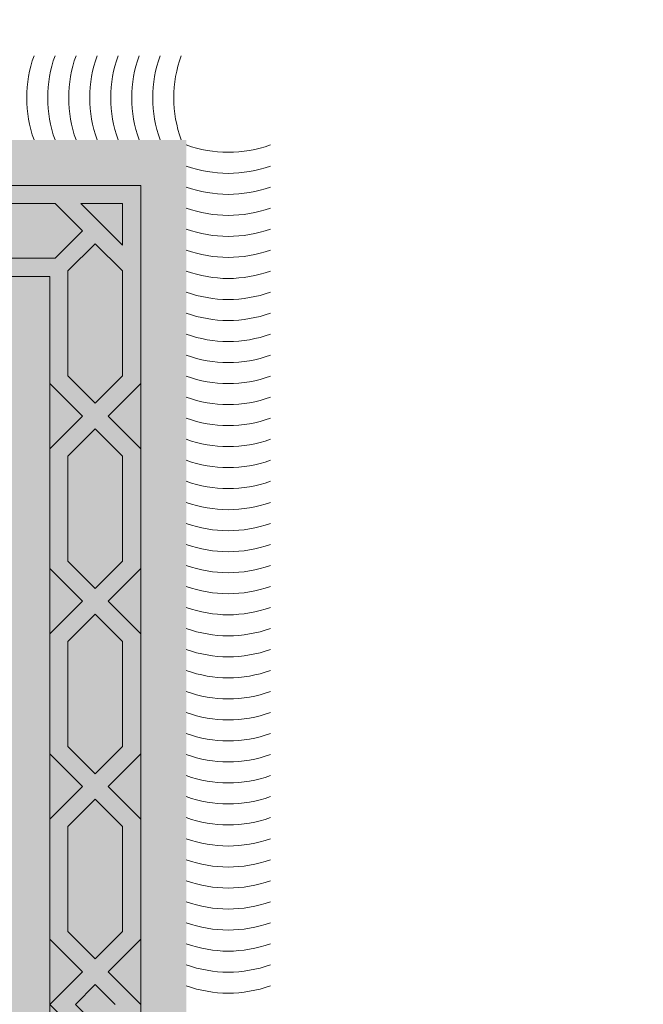
# Model space of a CAD drawing. Units: inches. Extents: x 844 to 2234, y 346 to 1084.
# Tile 22 of 93: x 1127.54 to 1136.28, y 696.22 to 710.02. Entities that reach past the tile are written whole.
import ezdxf

# ---------------------------------------------------------------- set-up
doc = ezdxf.new("R2010")
doc.units = ezdxf.units.IN
doc.header["$MEASUREMENT"] = 0
for name, color, linetype, lineweight in [('A-ANNO-DIMS', 2, 'Continuous', 18), ('furniture', 8, 'Continuous', 18), ('RA-AP-01$0$INT', 35, 'Continuous', 5)]:
    doc.layers.add(name, color=color, linetype=linetype, lineweight=lineweight)
doc.layers.add('RA-AP-01$0$FURN', color=3, linetype='Continuous')
doc.styles.get("Standard").update_dxf_attribs({"font": 'arial.ttf'})
doc.dimstyles.get("Standard").update_dxf_attribs({"dimtxt": 6, "dimasz": 3, "dimexe": 0.18, "dimexo": 0.0625, "dimgap": 0.09, "dimtad": 0, "dimtih": 1, "dimtoh": 1, "dimdec": 1, "dimzin": 0, "dimdsep": 46, "dimlunit": 3, "dimtxsty": 'Standard', "dimblk": 'ARCHTICK', "dimcen": 0.09, "dimadec": 0, "dimazin": 0, "dimtfac": 1, "dimtdec": 1, "dimtofl": 0, "dimtmove": 0, "dimatfit": 3, "dimfxl": 1, "dimtolj": 1, "dimtzin": 0, "dimarcsym": 0})

# ---------------------------------------------------------------- blocks, each defined once
blk = doc.blocks.new('A$C18D01794')
at = {"layer": 'RA-AP-01$0$INT'}
h = blk.add_hatch(color=256, dxfattribs=at)
h.paths.add_polyline_path([(4.3552, -6.1567), (4.3552, -8.0567), (5.4552, -8.0567), (5.4552, -6.1567)])
h.paths.add_polyline_path([(4.4052, -8.0067), (4.4052, -6.2067), (5.4052, -6.2067), (5.4052, -8.0067)], flags=16)
h = blk.add_hatch(color=256, dxfattribs=at)
h.paths.add_polyline_path([(4.4693, -7.0709), (4.5052, -7.035), (4.5052, -7.1067)])
h.paths.add_polyline_path([(4.4552, -7.085), (4.4769, -7.1067), (4.4335, -7.1067)])
h.paths.add_polyline_path([(4.4052, -7.035), (4.4411, -7.0709), (4.4052, -7.1067)])
h.paths.add_polyline_path([(4.4252, -6.9115), (4.4552, -6.8815), (4.4852, -6.9115), (4.4852, -7.0267), (4.4552, -7.0567), (4.4252, -7.0267)])
h.paths.add_polyline_path([(4.5052, -6.8315), (4.5052, -6.9032), (4.4693, -6.8673)])
h.paths.add_polyline_path([(4.4252, -6.7079), (4.4552, -6.6779), (4.4852, -6.7079), (4.4852, -6.8232), (4.4552, -6.8532), (4.4252, -6.8232)])
h.paths.add_polyline_path([(4.4252, -6.5044), (4.4552, -6.4744), (4.4852, -6.5044), (4.4852, -6.6196), (4.4552, -6.6496), (4.4252, -6.6196)])
h.paths.add_polyline_path([(4.4693, -6.6638), (4.5052, -6.6279), (4.5052, -6.6996)])
h.paths.add_polyline_path([(4.4052, -6.6279), (4.4411, -6.6638), (4.4052, -6.6996)])
h.paths.add_polyline_path([(4.4052, -6.4244), (4.4411, -6.4602), (4.4052, -6.4961)])
h.paths.add_polyline_path([(4.4693, -6.4602), (4.5052, -6.4244), (4.5052, -6.4961)])
h.paths.add_polyline_path([(4.4252, -6.3009), (4.4552, -6.2709), (4.4852, -6.3009), (4.4852, -6.4161), (4.4552, -6.4461), (4.4252, -6.4161)])
h.paths.add_polyline_path([(4.4252, -6.2267), (4.4711, -6.2267), (4.4252, -6.2726)])
h.paths.add_polyline_path([(4.4993, -6.2267), (4.6361, -6.2267), (4.6661, -6.2567), (4.6361, -6.2867), (4.4993, -6.2867), (4.4693, -6.2567)])
h.paths.add_polyline_path([(4.6802, -6.2709), (4.7161, -6.3067), (4.6443, -6.3067)])
h.paths.add_polyline_path([(4.6443, -6.2067), (4.7161, -6.2067), (4.6802, -6.2426)])
h.paths.add_polyline_path([(4.7243, -6.2267), (4.8611, -6.2267), (4.8911, -6.2567), (4.8611, -6.2867), (4.7243, -6.2867), (4.6943, -6.2567)])
h.paths.add_polyline_path([(4.9052, -6.2709), (4.9411, -6.3067), (4.8693, -6.3067)])
h.paths.add_polyline_path([(4.8693, -6.2067), (4.9411, -6.2067), (4.9052, -6.2426)])
h.paths.add_polyline_path([(4.9493, -6.2267), (5.0861, -6.2267), (5.1161, -6.2567), (5.0861, -6.2867), (4.9493, -6.2867), (4.9193, -6.2567)])
h.paths.add_polyline_path([(5.1302, -6.2709), (5.1661, -6.3067), (5.0943, -6.3067)])
h.paths.add_polyline_path([(5.0943, -6.2067), (5.1661, -6.2067), (5.1302, -6.2426)])
h.paths.add_polyline_path([(5.1743, -6.2267), (5.3111, -6.2267), (5.3411, -6.2567), (5.3111, -6.2867), (5.1743, -6.2867), (5.1443, -6.2567)])
h.paths.add_polyline_path([(5.3252, -6.3009), (5.3552, -6.2709), (5.3852, -6.3009), (5.3852, -6.4161), (5.3552, -6.4461), (5.3252, -6.4161)])
h.paths.add_polyline_path([(5.3393, -6.2267), (5.3852, -6.2267), (5.3852, -6.2726)])
h.paths.add_polyline_path([(5.3252, -6.5044), (5.3552, -6.4744), (5.3852, -6.5044), (5.3852, -6.6196), (5.3552, -6.6496), (5.3252, -6.6196)])
h.paths.add_polyline_path([(5.3052, -6.4244), (5.3411, -6.4602), (5.3052, -6.4961)])
h.paths.add_polyline_path([(5.3693, -6.4602), (5.4052, -6.4244), (5.4052, -6.4961)])
h.paths.add_polyline_path([(5.4052, -6.6279), (5.4052, -6.6996), (5.3693, -6.6638)])
h.paths.add_polyline_path([(5.3052, -6.6279), (5.3411, -6.6638), (5.3052, -6.6996)])
h.paths.add_polyline_path([(5.3252, -6.7079), (5.3552, -6.6779), (5.3852, -6.7079), (5.3852, -6.8232), (5.3552, -6.8532), (5.3252, -6.8232)])
h.paths.add_polyline_path([(5.3052, -6.8315), (5.3411, -6.8673), (5.3052, -6.9032)])
h.paths.add_polyline_path([(5.3252, -6.9115), (5.3552, -6.8815), (5.3852, -6.9115), (5.3852, -7.0267), (5.3552, -7.0567), (5.3252, -7.0267)])
h.paths.add_polyline_path([(5.4046, -6.8321, 0.001218), (5.4052, -6.8323), (5.4052, -6.9032), (5.3693, -6.8673)])
h.paths.add_polyline_path([(5.3693, -7.0709), (5.4052, -7.035), (5.4052, -7.1067)])
h.paths.add_polyline_path([(5.3552, -7.085), (5.3769, -7.1067), (5.3335, -7.1067)])
h.paths.add_polyline_path([(5.3052, -7.035), (5.3411, -7.0709), (5.3052, -7.1067)])
h = blk.add_hatch(color=256, dxfattribs=at)
h.paths.add_polyline_path([(4.5052, -6.6279), (4.4693, -6.6638), (4.5052, -6.6996), (4.5052, -6.8315), (4.4693, -6.8673), (4.5052, -6.9032), (4.5052, -7.035), (4.4693, -7.0709), (4.5052, -7.1067), (4.4769, -7.1067), (4.4552, -7.085), (4.4335, -7.1067), (4.4052, -7.1067), (4.4411, -7.0709), (4.4052, -7.035), (4.4052, -6.9032), (4.4411, -6.8673), (4.4052, -6.8315), (4.4052, -6.6996), (4.4411, -6.6638), (4.4052, -6.6279), (4.4052, -6.4961), (4.4411, -6.4602), (4.4052, -6.4244), (4.4052, -6.2067), (4.6443, -6.2067), (4.6802, -6.2426), (4.7161, -6.2067), (4.8693, -6.2067), (4.9052, -6.2426), (4.9411, -6.2067), (5.0943, -6.2067), (5.1302, -6.2426), (5.1661, -6.2067), (5.4052, -6.2067), (5.4052, -6.4244), (5.3693, -6.4602), (5.4052, -6.4961), (5.4052, -6.6279), (5.3693, -6.6638), (5.4052, -6.6996), (5.4052, -6.8315), (5.3693, -6.8673), (5.4052, -6.9032), (5.4052, -7.035), (5.3693, -7.0709), (5.4052, -7.1067), (5.3769, -7.1067), (5.3552, -7.085), (5.3335, -7.1067), (5.3052, -7.1067), (5.3411, -7.0709), (5.3052, -7.035), (5.3052, -6.9032), (5.3411, -6.8673), (5.3052, -6.8315), (5.3052, -6.6996), (5.3411, -6.6638), (5.3052, -6.6279), (5.3052, -6.4961), (5.3411, -6.4602), (5.3052, -6.4244), (5.3052, -6.3067), (5.1661, -6.3067), (5.1302, -6.2709), (5.0943, -6.3067), (4.9411, -6.3067), (4.9052, -6.2709), (4.8693, -6.3067), (4.7161, -6.3067), (4.6802, -6.2709), (4.6443, -6.3067), (4.5052, -6.3067), (4.5052, -6.4244), (4.4693, -6.4602), (4.5052, -6.4961)])
h.paths.add_polyline_path([(4.4852, -6.5044), (4.4552, -6.4744), (4.4252, -6.5044), (4.4252, -6.6196), (4.4552, -6.6496), (4.4852, -6.6196)], flags=16)
h.paths.add_polyline_path([(4.4552, -6.4461), (4.4852, -6.4161), (4.4852, -6.3009), (4.4552, -6.2709), (4.4252, -6.3009), (4.4252, -6.4161)], flags=16)
h.paths.add_polyline_path([(4.4552, -6.6779), (4.4252, -6.7079), (4.4252, -6.8232), (4.4552, -6.8532), (4.4852, -6.8232), (4.4852, -6.7079)], flags=16)
h.paths.add_polyline_path([(4.4993, -6.2867), (4.6361, -6.2867), (4.6661, -6.2567), (4.6361, -6.2267), (4.4993, -6.2267), (4.4693, -6.2567)], flags=16)
h.paths.add_polyline_path([(4.4252, -6.2726), (4.4711, -6.2267), (4.4252, -6.2267)], flags=16)
h.paths.add_polyline_path([(4.4552, -6.8815), (4.4252, -6.9115), (4.4252, -7.0267), (4.4552, -7.0567), (4.4852, -7.0267), (4.4852, -6.9115)], flags=16)
h.paths.add_polyline_path([(4.7243, -6.2867), (4.8611, -6.2867), (4.8911, -6.2567), (4.8611, -6.2267), (4.7243, -6.2267), (4.6943, -6.2567)], flags=16)
h.paths.add_polyline_path([(4.9193, -6.2567), (4.9493, -6.2867), (5.0861, -6.2867), (5.1161, -6.2567), (5.0861, -6.2267), (4.9493, -6.2267)], flags=16)
h.paths.add_polyline_path([(5.1443, -6.2567), (5.1743, -6.2867), (5.3111, -6.2867), (5.3411, -6.2567), (5.3111, -6.2267), (5.1743, -6.2267)], flags=16)
h.paths.add_polyline_path([(5.3252, -6.6196), (5.3552, -6.6496), (5.3852, -6.6196), (5.3852, -6.5044), (5.3552, -6.4744), (5.3252, -6.5044)], flags=16)
h.paths.add_polyline_path([(5.3252, -6.4161), (5.3552, -6.4461), (5.3852, -6.4161), (5.3852, -6.3009), (5.3552, -6.2709), (5.3252, -6.3009)], flags=16)
h.paths.add_polyline_path([(5.3252, -6.7079), (5.3252, -6.8232), (5.3552, -6.8532), (5.3852, -6.8232), (5.3852, -6.7079), (5.3552, -6.6779)], flags=16)
h.paths.add_polyline_path([(5.3252, -6.9115), (5.3252, -7.0267), (5.3552, -7.0567), (5.3852, -7.0267), (5.3852, -6.9115), (5.3552, -6.8815)], flags=16)
h.paths.add_polyline_path([(5.3393, -6.2267), (5.3852, -6.2726), (5.3852, -6.2267)], flags=16)
for points in [[(4.5052, -6.3067), (5.3052, -6.3067), (5.3052, -7.1067), (5.2552, -7.1067), (5.2552, -6.3567), (4.5552, -6.3567), (4.5552, -7.1067), (4.5052, -7.1067)], [(4.5052, -7.9067), (5.3052, -7.9067), (5.3052, -7.1067), (5.2552, -7.1067), (5.2552, -7.8567), (4.5552, -7.8567), (4.5552, -7.1067), (4.5052, -7.1067)]]:
    blk.add_hatch(color=256, dxfattribs=at).paths.add_polyline_path(points)
h = blk.add_hatch(color=256, dxfattribs=at)
h.paths.add_polyline_path([(4.5052, -7.5855), (4.4693, -7.5496), (4.5052, -7.5138), (4.5052, -7.382), (4.4693, -7.3461), (4.5052, -7.3102), (4.5052, -7.1784), (4.4693, -7.1426), (4.5052, -7.1067), (4.4769, -7.1067), (4.4552, -7.1284), (4.4335, -7.1067), (4.4052, -7.1067), (4.4411, -7.1426), (4.4052, -7.1784), (4.4052, -7.3102), (4.4411, -7.3461), (4.4052, -7.382), (4.4052, -7.5138), (4.4411, -7.5496), (4.4052, -7.5855), (4.4052, -7.7173), (4.4411, -7.7532), (4.4052, -7.789), (4.4052, -8.0067), (4.6443, -8.0067), (4.6802, -7.9709), (4.7161, -8.0067), (4.8693, -8.0067), (4.9052, -7.9709), (4.9411, -8.0067), (5.0943, -8.0067), (5.1302, -7.9709), (5.1661, -8.0067), (5.4052, -8.0067), (5.4052, -7.789), (5.3693, -7.7532), (5.4052, -7.7173), (5.4052, -7.5855), (5.3693, -7.5496), (5.4052, -7.5138), (5.4052, -7.382), (5.3693, -7.3461), (5.4052, -7.3102), (5.4052, -7.1784), (5.3693, -7.1426), (5.4052, -7.1067), (5.3769, -7.1067), (5.3552, -7.1284), (5.3335, -7.1067), (5.3052, -7.1067), (5.3411, -7.1426), (5.3052, -7.1784), (5.3052, -7.3102), (5.3411, -7.3461), (5.3052, -7.382), (5.3052, -7.5138), (5.3411, -7.5496), (5.3052, -7.5855), (5.3052, -7.7173), (5.3411, -7.7532), (5.3052, -7.789), (5.3052, -7.9067), (5.1661, -7.9067), (5.1302, -7.9426), (5.0943, -7.9067), (4.9411, -7.9067), (4.9052, -7.9426), (4.8693, -7.9067), (4.7161, -7.9067), (4.6802, -7.9426), (4.6443, -7.9067), (4.5052, -7.9067), (4.5052, -7.789), (4.4693, -7.7532), (4.5052, -7.7173)])
h.paths.add_polyline_path([(4.4852, -7.709), (4.4552, -7.739), (4.4252, -7.709), (4.4252, -7.5938), (4.4552, -7.5638), (4.4852, -7.5938)], flags=16)
h.paths.add_polyline_path([(4.4552, -7.7673), (4.4852, -7.7973), (4.4852, -7.9126), (4.4552, -7.9426), (4.4252, -7.9126), (4.4252, -7.7973)], flags=16)
h.paths.add_polyline_path([(4.4552, -7.5355), (4.4252, -7.5055), (4.4252, -7.3902), (4.4552, -7.3602), (4.4852, -7.3902), (4.4852, -7.5055)], flags=16)
h.paths.add_polyline_path([(4.4993, -7.9267), (4.6361, -7.9267), (4.6661, -7.9567), (4.6361, -7.9867), (4.4993, -7.9867), (4.4693, -7.9567)], flags=16)
h.paths.add_polyline_path([(4.4252, -7.9409), (4.4711, -7.9867), (4.4252, -7.9867)], flags=16)
h.paths.add_polyline_path([(4.4552, -7.332), (4.4252, -7.302), (4.4252, -7.1867), (4.4552, -7.1567), (4.4852, -7.1867), (4.4852, -7.302)], flags=16)
h.paths.add_polyline_path([(4.7243, -7.9267), (4.8611, -7.9267), (4.8911, -7.9567), (4.8611, -7.9867), (4.7243, -7.9867), (4.6943, -7.9567)], flags=16)
h.paths.add_polyline_path([(4.9193, -7.9567), (4.9493, -7.9267), (5.0861, -7.9267), (5.1161, -7.9567), (5.0861, -7.9867), (4.9493, -7.9867)], flags=16)
h.paths.add_polyline_path([(5.1443, -7.9567), (5.1743, -7.9267), (5.3111, -7.9267), (5.3411, -7.9567), (5.3111, -7.9867), (5.1743, -7.9867)], flags=16)
h.paths.add_polyline_path([(5.3252, -7.5938), (5.3552, -7.5638), (5.3852, -7.5938), (5.3852, -7.709), (5.3552, -7.739), (5.3252, -7.709)], flags=16)
h.paths.add_polyline_path([(5.3252, -7.7973), (5.3552, -7.7673), (5.3852, -7.7973), (5.3852, -7.9126), (5.3552, -7.9426), (5.3252, -7.9126)], flags=16)
h.paths.add_polyline_path([(5.3252, -7.5055), (5.3252, -7.3902), (5.3552, -7.3602), (5.3852, -7.3902), (5.3852, -7.5055), (5.3552, -7.5355)], flags=16)
h.paths.add_polyline_path([(5.3252, -7.302), (5.3252, -7.1867), (5.3552, -7.1567), (5.3852, -7.1867), (5.3852, -7.302), (5.3552, -7.332)], flags=16)
h.paths.add_polyline_path([(5.3393, -7.9867), (5.3852, -7.9409), (5.3852, -7.9867)], flags=16)
h = blk.add_hatch(color=256, dxfattribs=at)
h.paths.add_polyline_path([(4.4693, -7.1426), (4.5052, -7.1784), (4.5052, -7.1067)])
h.paths.add_polyline_path([(4.4552, -7.1284), (4.4769, -7.1067), (4.4335, -7.1067)])
h.paths.add_polyline_path([(4.4052, -7.1784), (4.4411, -7.1426), (4.4052, -7.1067)])
h.paths.add_polyline_path([(4.4252, -7.302), (4.4552, -7.332), (4.4852, -7.302), (4.4852, -7.1867), (4.4552, -7.1567), (4.4252, -7.1867)])
h.paths.add_polyline_path([(4.5052, -7.382), (4.5052, -7.3102), (4.4693, -7.3461)])
h.paths.add_polyline_path([(4.4252, -7.5055), (4.4552, -7.5355), (4.4852, -7.5055), (4.4852, -7.3902), (4.4552, -7.3602), (4.4252, -7.3902)])
h.paths.add_polyline_path([(4.4252, -7.709), (4.4552, -7.739), (4.4852, -7.709), (4.4852, -7.5938), (4.4552, -7.5638), (4.4252, -7.5938)])
h.paths.add_polyline_path([(4.4693, -7.5496), (4.5052, -7.5855), (4.5052, -7.5138)])
h.paths.add_polyline_path([(4.4052, -7.5855), (4.4411, -7.5496), (4.4052, -7.5138)])
h.paths.add_polyline_path([(4.4052, -7.789), (4.4411, -7.7532), (4.4052, -7.7173)])
h.paths.add_polyline_path([(4.4693, -7.7532), (4.5052, -7.789), (4.5052, -7.7173)])
h.paths.add_polyline_path([(4.4252, -7.9126), (4.4552, -7.9426), (4.4852, -7.9126), (4.4852, -7.7973), (4.4552, -7.7673), (4.4252, -7.7973)])
h.paths.add_polyline_path([(4.4252, -7.9867), (4.4711, -7.9867), (4.4252, -7.9409)])
h.paths.add_polyline_path([(4.4993, -7.9867), (4.6361, -7.9867), (4.6661, -7.9567), (4.6361, -7.9267), (4.4993, -7.9267), (4.4693, -7.9567)])
h.paths.add_polyline_path([(4.6802, -7.9426), (4.7161, -7.9067), (4.6443, -7.9067)])
h.paths.add_polyline_path([(4.6443, -8.0067), (4.7161, -8.0067), (4.6802, -7.9709)])
h.paths.add_polyline_path([(4.7243, -7.9867), (4.8611, -7.9867), (4.8911, -7.9567), (4.8611, -7.9267), (4.7243, -7.9267), (4.6943, -7.9567)])
h.paths.add_polyline_path([(4.9052, -7.9426), (4.9411, -7.9067), (4.8693, -7.9067)])
h.paths.add_polyline_path([(4.8693, -8.0067), (4.9411, -8.0067), (4.9052, -7.9709)])
h.paths.add_polyline_path([(4.9493, -7.9867), (5.0861, -7.9867), (5.1161, -7.9567), (5.0861, -7.9267), (4.9493, -7.9267), (4.9193, -7.9567)])
h.paths.add_polyline_path([(5.1302, -7.9426), (5.1661, -7.9067), (5.0943, -7.9067)])
h.paths.add_polyline_path([(5.0943, -8.0067), (5.1661, -8.0067), (5.1302, -7.9709)])
h.paths.add_polyline_path([(5.1743, -7.9867), (5.3111, -7.9867), (5.3411, -7.9567), (5.3111, -7.9267), (5.1743, -7.9267), (5.1443, -7.9567)])
h.paths.add_polyline_path([(5.3252, -7.9126), (5.3552, -7.9426), (5.3852, -7.9126), (5.3852, -7.7973), (5.3552, -7.7673), (5.3252, -7.7973)])
h.paths.add_polyline_path([(5.3393, -7.9867), (5.3852, -7.9867), (5.3852, -7.9409)])
h.paths.add_polyline_path([(5.3252, -7.709), (5.3552, -7.739), (5.3852, -7.709), (5.3852, -7.5938), (5.3552, -7.5638), (5.3252, -7.5938)])
h.paths.add_polyline_path([(5.3052, -7.789), (5.3411, -7.7532), (5.3052, -7.7173)])
h.paths.add_polyline_path([(5.3693, -7.7532), (5.4052, -7.789), (5.4052, -7.7173)])
h.paths.add_polyline_path([(5.4052, -7.5855), (5.4052, -7.5138), (5.3693, -7.5496)])
h.paths.add_polyline_path([(5.3052, -7.5855), (5.3411, -7.5496), (5.3052, -7.5138)])
h.paths.add_polyline_path([(5.3252, -7.5055), (5.3552, -7.5355), (5.3852, -7.5055), (5.3852, -7.3902), (5.3552, -7.3602), (5.3252, -7.3902)])
h.paths.add_polyline_path([(5.3052, -7.382), (5.3411, -7.3461), (5.3052, -7.3102)])
h.paths.add_polyline_path([(5.3252, -7.302), (5.3552, -7.332), (5.3852, -7.302), (5.3852, -7.1867), (5.3552, -7.1567), (5.3252, -7.1867)])
h.paths.add_polyline_path([(5.4046, -7.3813, -0.001218), (5.4052, -7.3811), (5.4052, -7.3102), (5.3693, -7.3461)])
h.paths.add_polyline_path([(5.3693, -7.1426), (5.4052, -7.1784), (5.4052, -7.1067)])
h.paths.add_polyline_path([(5.3552, -7.1284), (5.3769, -7.1067), (5.3335, -7.1067)])
h.paths.add_polyline_path([(5.3052, -7.1784), (5.3411, -7.1426), (5.3052, -7.1067)])
for p, q in [((5.3411, -7.0709), (5.3052, -7.1067)), ((5.3552, -7.085), (5.3335, -7.1067)), ((5.3411, -7.1426), (5.3052, -7.1067)), ((5.3552, -7.1284), (5.3335, -7.1067)), ((5.3552, -7.1284), (5.3769, -7.1067)), ((5.3693, -7.1426), (5.4052, -7.1067)), ((5.3052, -7.1784), (5.3411, -7.1426)), ((5.4052, -7.1784), (5.3693, -7.1426)), ((5.3252, -7.1867), (5.3552, -7.1567)), ((5.3852, -7.1867), (5.3552, -7.1567)), ((5.3252, -7.302), (5.3252, -7.1867)), ((5.3852, -7.302), (5.3852, -7.1867)), ((5.3252, -7.302), (5.3552, -7.332)), ((5.3852, -7.302), (5.3552, -7.332)), ((5.3052, -7.3102), (5.3411, -7.3461)), ((5.4052, -7.3102), (5.3693, -7.3461)), ((5.3052, -7.382), (5.3411, -7.3461)), ((5.4052, -7.382), (5.3693, -7.3461)), ((5.3252, -7.3902), (5.3552, -7.3602)), ((5.3852, -7.3902), (5.3552, -7.3602)), ((5.3252, -7.3902), (5.3252, -7.5055)), ((5.3852, -7.3902), (5.3852, -7.5055)), ((5.3252, -7.5055), (5.3552, -7.5355)), ((5.3852, -7.5055), (5.3552, -7.5355)), ((5.3052, -7.5138), (5.3411, -7.5496)), ((5.4052, -7.5138), (5.3693, -7.5496)), ((5.3052, -7.5855), (5.3411, -7.5496)), ((5.4052, -7.5855), (5.3693, -7.5496)), ((5.3252, -7.5938), (5.3552, -7.5638)), ((5.3852, -7.5938), (5.3552, -7.5638)), ((5.3252, -7.5938), (5.3252, -7.709)), ((5.3852, -7.5938), (5.3852, -7.709)), ((5.3252, -7.709), (5.3552, -7.739)), ((5.3852, -7.709), (5.3552, -7.739)), ((5.3052, -7.7173), (5.3411, -7.7532)), ((5.4052, -7.7173), (5.3693, -7.7532)), ((5.3411, -7.7532), (5.3052, -7.789)), ((5.3693, -7.7532), (5.4052, -7.789)), ((5.3552, -7.7673), (5.3252, -7.7973)), ((5.3552, -7.7673), (5.3852, -7.7973)), ((5.3252, -7.9126), (5.3252, -7.7973)), ((5.3852, -7.7973), (5.3852, -7.9126)), ((5.3252, -7.9126), (5.3552, -7.9426)), ((5.3852, -7.9126), (5.3552, -7.9426)), ((5.1743, -7.9267), (5.3111, -7.9267)), ((5.3111, -7.9267), (5.3411, -7.9567)), ((5.3393, -7.9867), (5.3852, -7.9409)), ((5.3852, -7.9409), (5.3852, -7.9867)), ((5.3111, -7.9867), (5.3411, -7.9567)), ((5.1743, -7.9867), (5.3111, -7.9867)), ((5.3393, -7.9867), (5.3852, -7.9867))]:
    blk.add_line(p, q, dxfattribs=at)
for points in [[(5.4052, -7.1067), (5.4052, -6.2067)], [(5.3052, -7.1067), (5.3052, -6.3067), (4.5052, -6.3067), (4.5052, -7.1067)], [(5.4052, -8.0067), (4.4052, -8.0067), (4.4052, -7.1067)], [(5.3052, -7.1067), (5.3052, -7.9067), (4.5052, -7.9067), (4.5052, -7.1067)], [(5.4052, -7.1067), (5.4052, -8.0067)]]:
    blk.add_lwpolyline(points, dxfattribs=at)
for centre, start, end in [((5.5014, -7.2554), 70.2038, 109.7962), ((5.5014, -7.2785), 70.2038, 109.7962), ((5.5014, -7.3016), 70.2038, 109.7962), ((5.5014, -7.3247), 70.2038, 109.7962), ((5.5014, -7.3478), 70.2038, 109.7962), ((5.5014, -7.3709), 70.2038, 109.7962), ((5.5014, -7.394), 70.2038, 109.7962), ((5.5014, -7.4171), 70.2038, 109.7962), ((5.5014, -7.4402), 70.2038, 109.7962), ((5.5014, -7.4633), 70.2038, 109.7962), ((5.5014, -7.4864), 70.2038, 109.7962), ((5.5014, -7.5095), 70.2038, 109.7962), ((5.5014, -7.5326), 70.2038, 109.7962), ((5.5014, -7.5557), 70.2038, 109.7962), ((5.5014, -7.5788), 70.2038, 109.7962), ((5.5014, -7.6019), 70.2038, 109.7962), ((5.5014, -7.625), 70.2038, 109.7962), ((5.5014, -7.6481), 70.2038, 109.7962), ((5.5014, -7.6712), 70.2038, 109.7962), ((5.5014, -7.6712), 70.2038, 109.7962), ((5.5014, -7.6943), 70.2038, 109.7962), ((5.5014, -7.7174), 70.2038, 109.7962), ((5.5014, -7.7405), 70.2038, 109.7962), ((5.5014, -7.7636), 70.2038, 109.7962), ((5.5014, -7.7867), 70.2038, 109.7962), ((5.5014, -7.8098), 70.2038, 109.7962), ((5.5014, -7.8329), 70.2038, 109.7962), ((5.5014, -7.856), 70.2038, 109.7962), ((5.5014, -7.8791), 70.2038, 109.7962), ((5.5014, -7.9022), 70.2038, 109.7962), ((5.5014, -7.9253), 70.2038, 109.7962), ((5.5014, -7.9484), 70.2038, 109.7962), ((5.5014, -7.9715), 70.2038, 109.7962), ((5.5014, -7.9946), 70.2038, 109.7962), ((5.5014, -8.0177), 70.2038, 109.7962), ((5.5014, -8.0408), 70.2038, 109.7962), ((5.5014, -8.0639), 70.2038, 109.7962), ((5.5014, -8.087), 70.2038, 109.7962), ((5.5014, -8.1101), 70.2038, 109.7962), ((5.5014, -8.1332), 70.2038, 109.7962), ((5.5014, -8.1563), 70.2038, 109.7962), ((5.5014, -8.1794), 70.2038, 109.7962), ((5.4162, -8.1029), 160.2038, 199.7962), ((5.4393, -8.1029), 160.2038, 199.7962), ((5.4624, -8.1029), 160.2038, 199.7962), ((5.4855, -8.1029), 160.2038, 199.7962), ((5.5086, -8.1029), 160.2038, 199.7962), ((5.5317, -8.1029), 160.2038, 199.7962), ((5.5548, -8.1029), 160.2038, 199.7962), ((5.5779, -8.1029), 160.2038, 199.7962)]:
    blk.add_arc(centre, 0.1364, start, end, dxfattribs=at)
blk = doc.blocks.new('A$C5D2F253E')
at = {"layer": 'RA-AP-01$0$FURN', "xscale": -0.7999999999883585, "yscale": 0.7999999999883585, "zscale": 0.8, "rotation": 90}
blk.add_blockref('A$C18D01794', (-5.68776, 4.75792), dxfattribs=at)
blk = doc.blocks.new('_ArchTick')
at = {"color": 0, "linetype": 'ByBlock', "const_width": 0.15}
blk.add_lwpolyline([(-0.5, -0.5), (0.5, 0.5)], dxfattribs=at)
blk = doc.blocks.new('*D144')
at = {"layer": 'A-ANNO-DIMS', "color": 0, "lineweight": -2, "transparency": 16777216}
for p, q in [((1096.616, 439.373), (1096.616, 1074.743)), ((1143.116, 492.373), (1143.116, 1074.743)), ((1096.616, 1074.563), (1102.482, 1074.563)), ((1143.116, 1074.563), (1137.25, 1074.563))]:
    blk.add_line(p, q, dxfattribs=at)
at = {"layer": 'Defpoints', "color": 0, "transparency": 16777216}
for p in [(1143.116, 1074.563), (1143.116, 492.311), (1096.616, 439.311)]:
    blk.add_point(p, dxfattribs=at)
at = {"layer": 'A-ANNO-DIMS', "color": 0, "lineweight": -2, "transparency": 16777216, "xscale": 3, "yscale": 3, "zscale": 3, "rotation": 180}
blk.add_blockref('_ArchTick', (1096.616, 1074.563), dxfattribs=at)
at = {"layer": 'A-ANNO-DIMS', "color": 0, "lineweight": -2, "transparency": 16777216, "xscale": 3, "yscale": 3, "zscale": 3}
blk.add_blockref('_ArchTick', (1143.116, 1074.563), dxfattribs=at)
at = {"layer": 'A-ANNO-DIMS', "color": 0, "transparency": 16777216, "insert": (1119.866, 1074.563), "char_height": 6, "attachment_point": 5}
blk.add_mtext('\\A1;3\'-10 1/2"', dxfattribs=at)

msp = doc.modelspace()

# ---------------------------------------------------------------- block references
at = {"layer": 'furniture', "xscale": 15.94108302203742, "yscale": 15.94108302203742, "zscale": 15.94108302203742, "rotation": 90}
msp.add_blockref('A$C5D2F253E', (1136.148, 696.258), dxfattribs=at)

# ---------------------------------------------------------------- dimensions: what is measured, and where the dimension line sits
at = {"layer": 'A-ANNO-DIMS'}
dim = msp.add_linear_dim(base=(1143.116, 1074.563), p1=(1096.616, 439.311), p2=(1143.116, 492.311), dimstyle='Standard', override={"dimdec": 1, "dimlfac": 1, "dimrnd": 0, "dimzin": 1, "dimdsep": 46, "dimlunit": 4, "dimfrac": 2}, dxfattribs=at)
dim.commit()
dim.dimension.update_dxf_attribs({"geometry": '*D144', "text_midpoint": (1119.866, 1074.563)})

doc.saveas('drawing.dxf')
